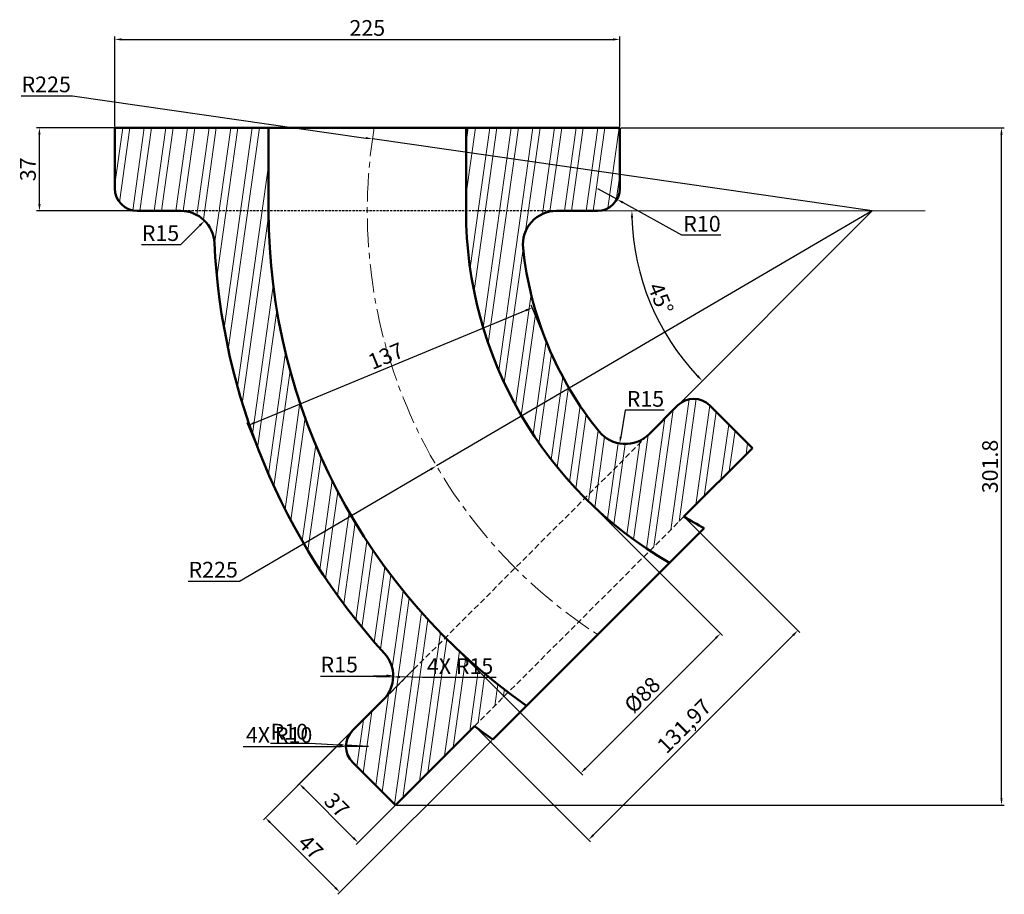
# Model space of a CAD drawing. Units: millimetres. Extents: x 315 to 754, y 170 to 559.
import ezdxf

# ---------------------------------------------------------------- set-up
doc = ezdxf.new("R2010")
doc.units = ezdxf.units.MM
doc.header["$LTSCALE"] = 0.4
doc.linetypes.add('CENTER', pattern=[50.8, 31.75, -6.35, 6.35, -6.35])
doc.linetypes.add('HIDDEN', pattern=[9.525, 6.35, -3.175])
for name, color, linetype, lineweight in [('M-CNTR', 4, 'CENTER', 18), ('M-CONS', 8, 'Continuous', 13), ('M-DIMS', 2, 'Continuous', 25), ('M-HATC', 9, 'Continuous', 18), ('M-HIDN', 3, 'HIDDEN', 25), ('M-OUTL', 7, 'Continuous', 50)]:
    doc.layers.add(name, color=color, linetype=linetype, lineweight=lineweight)
doc.styles.get("Standard").update_dxf_attribs({"font": 'arial.ttf'})
doc.dimstyles.new('ISO-25', dxfattribs={"dimtxt": 7, "dimasz": 3, "dimexe": 1.25, "dimexo": 0.625, "dimtad": 1, "dimtoh": 1, "dimtxsty": 'Standard', "dimcen": 2.5, "dimadec": 0, "dimazin": 0, "dimtfac": 1, "dimtmove": 0, "dimatfit": 3, "dimfxl": 1, "dimarcsym": 0})

# ---------------------------------------------------------------- blocks, each defined once
blk = doc.blocks.new('*D1')
at = {"layer": 'Defpoints', "color": 0, "ltscale": 0.4, "transparency": 16777216}
for p in [(582.55, 550.47), (357.55, 511.07), (582.55, 511.07)]:
    blk.add_point(p, dxfattribs=at)
at = {"layer": 'M-DIMS', "color": 0, "lineweight": -2, "ltscale": 0.4, "transparency": 16777216}
for p, q in [((357.55, 511.69), (357.55, 551.72)), ((360.55, 550.47), (579.55, 550.47)), ((582.55, 511.69), (582.55, 551.72))]:
    blk.add_line(p, q, dxfattribs=at)
at = {"layer": 'M-DIMS', "color": 0, "ltscale": 0.4, "transparency": 16777216}
for points in [[(360.55, 550.97), (360.55, 549.97), (357.55, 550.47)], [(579.55, 550.97), (579.55, 549.97), (582.55, 550.47)]]:
    blk.add_solid(points, dxfattribs=at)
at = {"layer": 'M-DIMS', "color": 0, "ltscale": 0.4, "transparency": 16777216, "insert": (470.05, 554.67), "char_height": 7, "attachment_point": 5}
blk.add_mtext('225', dxfattribs=at)
blk = doc.blocks.new('*D2')
at = {"layer": 'Defpoints', "color": 0, "ltscale": 0.4, "transparency": 16777216}
for p in [(323.97, 511.07), (377.23, 511.07), (377.23, 474.07)]:
    blk.add_point(p, dxfattribs=at)
at = {"layer": 'M-DIMS', "color": 0, "lineweight": -2, "ltscale": 0.4, "transparency": 16777216}
for p, q in [((376.61, 511.07), (322.72, 511.07)), ((323.97, 477.07), (323.97, 508.07)), ((376.61, 474.07), (322.72, 474.07))]:
    blk.add_line(p, q, dxfattribs=at)
at = {"layer": 'M-DIMS', "color": 0, "ltscale": 0.4, "transparency": 16777216}
for points in [[(323.47, 508.07), (324.47, 508.07), (323.97, 511.07)], [(323.47, 477.07), (324.47, 477.07), (323.97, 474.07)]]:
    blk.add_solid(points, dxfattribs=at)
at = {"layer": 'M-DIMS', "color": 0, "ltscale": 0.4, "transparency": 16777216, "insert": (319.76, 492.57), "char_height": 7, "attachment_point": 5, "rotation": 90}
blk.add_mtext('37', dxfattribs=at)
blk = doc.blocks.new('*D3')
at = {"layer": 'Defpoints', "color": 0, "ltscale": 0.4, "transparency": 16777216}
for p in [(543.54, 430.9), (550.46, 414.18), (423.89, 361.75)]:
    blk.add_point(p, dxfattribs=at)
at = {"layer": 'M-DIMS', "color": 0, "lineweight": -2, "ltscale": 0.4, "transparency": 16777216}
for p, q in [((550.23, 414.75), (543.06, 432.05)), ((419.74, 379.62), (540.77, 429.75)), ((423.65, 362.33), (416.49, 379.63))]:
    blk.add_line(p, q, dxfattribs=at)
at = {"layer": 'M-DIMS', "color": 0, "ltscale": 0.4, "transparency": 16777216}
for points in [[(540.58, 430.21), (540.96, 429.29), (543.54, 430.9)], [(419.55, 380.08), (419.93, 379.16), (416.97, 378.47)]]:
    blk.add_solid(points, dxfattribs=at)
at = {"layer": 'M-DIMS', "color": 0, "ltscale": 0.4, "transparency": 16777216, "insert": (478.64, 408.57), "char_height": 7, "attachment_point": 5, "rotation": 22.5}
blk.add_mtext('137', dxfattribs=at)
blk = doc.blocks.new('*D4')
at = {"layer": 'Defpoints', "color": 0, "ltscale": 0.4, "transparency": 16777216}
for p in [(567.07, 346.08), (627.38, 285.76), (504.84, 283.86)]:
    blk.add_point(p, dxfattribs=at)
at = {"layer": 'M-DIMS', "color": 0, "lineweight": -2, "ltscale": 0.4, "transparency": 16777216}
for p, q in [((567.51, 345.64), (628.27, 284.88)), ((505.28, 283.41), (566.04, 222.65)), ((567.28, 225.66), (625.26, 283.64))]:
    blk.add_line(p, q, dxfattribs=at)
at = {"layer": 'M-DIMS', "color": 0, "ltscale": 0.4, "transparency": 16777216}
for points in [[(624.91, 284), (625.61, 283.29), (627.38, 285.76)], [(566.92, 226.01), (567.63, 225.31), (565.16, 223.54)]]:
    blk.add_solid(points, dxfattribs=at)
at = {"layer": 'M-DIMS', "color": 0, "ltscale": 0.4, "transparency": 16777216, "insert": (593.16, 257.76), "char_height": 7, "attachment_point": 5, "rotation": 45}
blk.add_mtext('%%C88', dxfattribs=at)
blk = doc.blocks.new('*D5')
at = {"layer": 'Defpoints', "color": 0, "ltscale": 0.4, "transparency": 16777216}
for p in [(611.14, 337.83), (661.89, 287.08), (517.83, 244.52)]:
    blk.add_point(p, dxfattribs=at)
at = {"layer": 'M-DIMS', "color": 0, "lineweight": -2, "ltscale": 0.4, "transparency": 16777216}
for p, q in [((611.59, 337.39), (662.78, 286.2)), ((570.7, 195.89), (659.77, 284.96)), ((518.27, 244.08), (569.46, 192.88))]:
    blk.add_line(p, q, dxfattribs=at)
at = {"layer": 'M-DIMS', "color": 0, "ltscale": 0.4, "transparency": 16777216}
for points in [[(659.42, 285.32), (660.13, 284.61), (661.89, 287.08)], [(570.35, 196.24), (571.05, 195.54), (568.58, 193.77)]]:
    blk.add_solid(points, dxfattribs=at)
at = {"layer": 'M-DIMS', "color": 0, "ltscale": 0.4, "transparency": 16777216, "insert": (611.82, 243.84), "char_height": 7, "attachment_point": 5, "rotation": 45}
blk.add_mtext('131,97', dxfattribs=at)
blk = doc.blocks.new('*D6')
at = {"layer": 'Defpoints', "color": 0, "ltscale": 0.4, "transparency": 16777216}
for p in [(477.17, 256.18), (503.33, 230.02), (465.92, 192.61)]:
    blk.add_point(p, dxfattribs=at)
at = {"layer": 'M-DIMS', "color": 0, "lineweight": -2, "ltscale": 0.4, "transparency": 16777216}
for p, q in [((476.73, 255.74), (438.87, 217.89)), ((502.89, 229.58), (465.03, 191.72)), ((441.88, 216.65), (463.8, 194.73))]:
    blk.add_line(p, q, dxfattribs=at)
at = {"layer": 'M-DIMS', "color": 0, "ltscale": 0.4, "transparency": 16777216}
for points in [[(442.23, 217), (441.52, 216.29), (439.75, 218.77)], [(464.15, 195.08), (463.44, 194.37), (465.92, 192.61)]]:
    blk.add_solid(points, dxfattribs=at)
at = {"layer": 'M-DIMS', "color": 0, "ltscale": 0.4, "transparency": 16777216, "insert": (455.81, 208.66), "char_height": 7, "attachment_point": 5, "rotation": 315}
blk.add_mtext('37', dxfattribs=at)
blk = doc.blocks.new('*D7')
at = {"layer": 'Defpoints', "color": 0, "ltscale": 0.4, "transparency": 16777216}
for p in [(492.7, 271.72), (525.94, 238.48), (424.63, 203.64)]:
    blk.add_point(p, dxfattribs=at)
at = {"layer": 'M-DIMS', "color": 0, "lineweight": -2, "ltscale": 0.4, "transparency": 16777216}
for p, q in [((492.26, 271.28), (423.74, 202.76)), ((525.49, 238.04), (456.98, 169.53)), ((455.74, 172.53), (426.75, 201.52))]:
    blk.add_line(p, q, dxfattribs=at)
at = {"layer": 'M-DIMS', "color": 0, "ltscale": 0.4, "transparency": 16777216}
for points in [[(427.1, 201.88), (426.4, 201.17), (424.63, 203.64)], [(456.09, 172.88), (455.39, 172.18), (457.86, 170.41)]]:
    blk.add_solid(points, dxfattribs=at)
at = {"layer": 'M-DIMS', "color": 0, "ltscale": 0.4, "transparency": 16777216, "insert": (444.16, 189.94), "char_height": 7, "attachment_point": 5, "rotation": 315}
blk.add_mtext('47', dxfattribs=at)
blk = doc.blocks.new('*D8')
at = {"layer": 'Defpoints', "color": 0, "ltscale": 0.4, "transparency": 16777216}
for p in [(572.55, 484.07), (581.3, 479.22)]:
    blk.add_point(p, dxfattribs=at)
at = {"layer": 'M-DIMS', "color": 0, "lineweight": -2, "ltscale": 0.4, "transparency": 16777216}
for p, q in [((572.55, 484.07), (581.3, 479.22)), ((610.17, 463.22), (583.92, 477.77)), ((627.5, 463.22), (610.17, 463.22))]:
    blk.add_line(p, q, dxfattribs=at)
at = {"layer": 'M-DIMS', "color": 0, "ltscale": 0.4, "transparency": 16777216}
blk.add_solid([(584.16, 478.2), (583.68, 477.33), (581.3, 479.22)], dxfattribs=at)
at = {"layer": 'M-DIMS', "color": 0, "ltscale": 0.4, "transparency": 16777216, "insert": (619.15, 467.42), "char_height": 7, "attachment_point": 5}
blk.add_mtext('R10', dxfattribs=at)
blk = doc.blocks.new('*D9')
at = {"layer": 'Defpoints', "color": 0, "ltscale": 0.4, "transparency": 16777216}
for p in [(584.95, 385.18), (582.45, 370.39)]:
    blk.add_point(p, dxfattribs=at)
at = {"layer": 'M-DIMS', "color": 0, "lineweight": -2, "ltscale": 0.4, "transparency": 16777216}
for p, q in [((584.96, 385.2), (582.95, 373.35)), ((602.36, 385.2), (584.96, 385.2))]:
    blk.add_line(p, q, dxfattribs=at)
at = {"layer": 'M-DIMS', "color": 0, "ltscale": 0.4, "transparency": 16777216}
blk.add_solid([(582.45, 373.43), (583.44, 373.27), (582.45, 370.39)], dxfattribs=at)
at = {"layer": 'M-DIMS', "color": 0, "ltscale": 0.4, "transparency": 16777216, "insert": (593.97, 389.39), "char_height": 7, "attachment_point": 5}
blk.add_mtext('R15', dxfattribs=at)
blk = doc.blocks.new('*D10')
at = {"layer": 'Defpoints', "color": 0, "ltscale": 0.4, "transparency": 16777216}
for p in [(397.52, 469.67), (386.92, 459.07)]:
    blk.add_point(p, dxfattribs=at)
at = {"layer": 'M-DIMS', "color": 0, "lineweight": -2, "ltscale": 0.4, "transparency": 16777216}
for p, q in [((386.91, 459.06), (395.4, 467.55)), ((369.5, 459.06), (386.91, 459.06))]:
    blk.add_line(p, q, dxfattribs=at)
at = {"layer": 'M-DIMS', "color": 0, "ltscale": 0.4, "transparency": 16777216}
blk.add_solid([(395.05, 467.91), (395.76, 467.2), (397.52, 469.67)], dxfattribs=at)
at = {"layer": 'M-DIMS', "color": 0, "ltscale": 0.4, "transparency": 16777216, "insert": (377.89, 463.26), "char_height": 7, "attachment_point": 5}
blk.add_mtext('R15', dxfattribs=at)
blk = doc.blocks.new('*D11')
at = {"layer": 'Defpoints', "color": 0, "ltscale": 0.4, "transparency": 16777216}
for p in [(695.05, 474.07), (500.86, 360.42)]:
    blk.add_point(p, dxfattribs=at)
at = {"layer": 'M-DIMS', "color": 0, "lineweight": -2, "ltscale": 0.4, "transparency": 16777216}
for p, q in [((695.05, 474.07), (500.86, 360.42)), ((413.12, 309.07), (498.27, 358.9)), ((390.28, 309.07), (413.12, 309.07))]:
    blk.add_line(p, q, dxfattribs=at)
at = {"layer": 'M-DIMS', "color": 0, "ltscale": 0.4, "transparency": 16777216}
blk.add_solid([(498.02, 359.33), (498.53, 358.47), (500.86, 360.42)], dxfattribs=at)
at = {"layer": 'M-DIMS', "color": 0, "ltscale": 0.4, "transparency": 16777216, "insert": (401.39, 313.27), "char_height": 7, "attachment_point": 5}
blk.add_mtext('R225', dxfattribs=at)
blk = doc.blocks.new('*D12')
at = {"layer": 'Defpoints', "color": 0, "ltscale": 0.4, "transparency": 16777216}
for p in [(466.56, 266.79), (481.56, 267)]:
    blk.add_point(p, dxfattribs=at)
at = {"layer": 'M-DIMS', "color": 0, "lineweight": -2, "ltscale": 0.4, "transparency": 16777216}
for p, q in [((449.14, 266.79), (466.55, 266.79)), ((466.55, 266.79), (478.56, 266.96))]:
    blk.add_line(p, q, dxfattribs=at)
at = {"layer": 'M-DIMS', "color": 0, "ltscale": 0.4, "transparency": 16777216}
blk.add_solid([(478.55, 267.46), (478.57, 266.46), (481.56, 267)], dxfattribs=at)
at = {"layer": 'M-DIMS', "color": 0, "ltscale": 0.4, "transparency": 16777216, "insert": (457.53, 270.99), "char_height": 7, "attachment_point": 5}
blk.add_mtext('R15', dxfattribs=at)
blk = doc.blocks.new('*D13')
at = {"layer": 'Defpoints', "color": 0, "ltscale": 0.4, "transparency": 16777216}
for p in [(460.56, 235.98), (470.55, 235.42)]:
    blk.add_point(p, dxfattribs=at)
at = {"layer": 'M-DIMS', "color": 0, "lineweight": -2, "ltscale": 0.4, "transparency": 16777216}
for p, q in [((426.96, 236.9), (444.29, 236.9)), ((444.29, 236.9), (457.57, 236.15)), ((470.55, 235.42), (460.56, 235.98))]:
    blk.add_line(p, q, dxfattribs=at)
at = {"layer": 'M-DIMS', "color": 0, "ltscale": 0.4, "transparency": 16777216}
blk.add_solid([(457.59, 236.65), (457.54, 235.65), (460.56, 235.98)], dxfattribs=at)
at = {"layer": 'M-DIMS', "color": 0, "ltscale": 0.4, "transparency": 16777216, "insert": (435.31, 241.1), "char_height": 7, "attachment_point": 5}
blk.add_mtext('R10', dxfattribs=at)
blk = doc.blocks.new('*D14')
at = {"layer": 'Defpoints', "color": 0, "ltscale": 0.4, "transparency": 16777216}
for p in [(563.45, 474.07), (695.05, 474.07), (718.61, 474.07), (591.59, 446.35), (602, 381.01)]:
    blk.add_point(p, dxfattribs=at)
at = {"layer": 'M-DIMS', "color": 0, "lineweight": -2, "ltscale": 0.4, "transparency": 16777216}
blk.add_arc((695.05, 474.07), 107.11, 181.6048, 223.3952, dxfattribs=at)
at = {"layer": 'M-DIMS', "color": 0, "ltscale": 0.4, "transparency": 16777216}
for points in [[(587.49, 471.06), (588.49, 471.07), (587.94, 474.07)], [(617.58, 400.83), (616.86, 400.13), (619.31, 398.33)]]:
    blk.add_solid(points, dxfattribs=at)
at = {"layer": 'M-DIMS', "color": 0, "ltscale": 0.4, "transparency": 16777216, "insert": (599.96, 434.68), "char_height": 7, "attachment_point": 5, "rotation": 292.5}
blk.add_mtext('45°', dxfattribs=at)
blk = doc.blocks.new('*D15')
at = {"layer": 'Defpoints', "color": 0, "ltscale": 0.4, "transparency": 16777216}
for p in [(582.55, 511.07), (752.61, 511.07), (482.57, 209.26)]:
    blk.add_point(p, dxfattribs=at)
at = {"layer": 'M-DIMS', "color": 0, "lineweight": -2, "ltscale": 0.4, "transparency": 16777216}
for p, q in [((583.18, 511.07), (753.86, 511.07)), ((752.61, 212.26), (752.61, 508.07)), ((483.19, 209.26), (753.86, 209.26))]:
    blk.add_line(p, q, dxfattribs=at)
at = {"layer": 'M-DIMS', "color": 0, "ltscale": 0.4, "transparency": 16777216}
for points in [[(752.11, 508.07), (753.11, 508.07), (752.61, 511.07)], [(752.11, 212.26), (753.11, 212.26), (752.61, 209.26)]]:
    blk.add_solid(points, dxfattribs=at)
at = {"layer": 'M-DIMS', "color": 0, "ltscale": 0.4, "transparency": 16777216, "insert": (748.41, 360.16), "char_height": 7, "attachment_point": 5, "rotation": 90}
blk.add_mtext('301.8', dxfattribs=at)
blk = doc.blocks.new('*D16')
at = {"layer": 'Defpoints', "color": 0, "ltscale": 0.4, "transparency": 16777216}
for p in [(466.56, 266.79), (481.56, 266.43)]:
    blk.add_point(p, dxfattribs=at)
at = {"layer": 'M-DIMS', "color": 0, "lineweight": -2, "ltscale": 0.4, "transparency": 16777216}
for p, q in [((466.56, 266.79), (481.56, 266.43)), ((494.7, 266.11), (484.56, 266.36)), ((527.43, 266.11), (494.7, 266.11))]:
    blk.add_line(p, q, dxfattribs=at)
at = {"layer": 'M-DIMS', "color": 0, "ltscale": 0.4, "transparency": 16777216}
blk.add_solid([(484.57, 266.86), (484.54, 265.86), (481.56, 266.43)], dxfattribs=at)
at = {"layer": 'M-DIMS', "color": 0, "ltscale": 0.4, "transparency": 16777216, "insert": (511.38, 270.31), "char_height": 7, "attachment_point": 5}
blk.add_mtext('4X R15', dxfattribs=at)
blk = doc.blocks.new('*D17')
at = {"layer": 'Defpoints', "color": 0, "ltscale": 0.4, "transparency": 16777216}
for p in [(460.55, 235.42), (470.55, 235.42)]:
    blk.add_point(p, dxfattribs=at)
at = {"layer": 'M-DIMS', "color": 0, "lineweight": -2, "ltscale": 0.4, "transparency": 16777216}
for p, q in [((414.75, 235.42), (447.4, 235.42)), ((447.4, 235.42), (457.55, 235.42)), ((470.55, 235.42), (460.55, 235.42))]:
    blk.add_line(p, q, dxfattribs=at)
at = {"layer": 'M-DIMS', "color": 0, "ltscale": 0.4, "transparency": 16777216}
blk.add_solid([(457.55, 235.92), (457.55, 234.92), (460.55, 235.42)], dxfattribs=at)
at = {"layer": 'M-DIMS', "color": 0, "ltscale": 0.4, "transparency": 16777216, "insert": (430.76, 239.62), "char_height": 7, "attachment_point": 5}
blk.add_mtext('4X R10', dxfattribs=at)
blk = doc.blocks.new('*D18')
at = {"layer": 'Defpoints', "color": 0, "ltscale": 0.4, "transparency": 16777216}
for p in [(472.34, 506.1), (695.05, 474.07)]:
    blk.add_point(p, dxfattribs=at)
at = {"layer": 'M-DIMS', "color": 0, "lineweight": -2, "ltscale": 0.4, "transparency": 16777216}
for p, q in [((315.88, 525.32), (338.72, 525.32)), ((338.72, 525.32), (469.37, 506.53)), ((695.05, 474.07), (472.34, 506.1))]:
    blk.add_line(p, q, dxfattribs=at)
at = {"layer": 'M-DIMS', "color": 0, "ltscale": 0.4, "transparency": 16777216}
blk.add_solid([(469.45, 507.02), (469.3, 506.03), (472.34, 506.1)], dxfattribs=at)
at = {"layer": 'M-DIMS', "color": 0, "ltscale": 0.4, "transparency": 16777216, "insert": (326.99, 529.52), "char_height": 7, "attachment_point": 5}
blk.add_mtext('R225', dxfattribs=at)

msp = doc.modelspace()

# ---------------------------------------------------------------- hatches: boundary and pattern name
at = {"layer": 'M-HATC', "ltscale": 0.4}
h = msp.add_hatch(dxfattribs=at)
h.set_pattern_fill('ANSI32', color=256, angle=37)
h.set_pattern_definition([(82, (-1722.207, -282.083), (-9.432303, 1.325624), []), (82, (-1718.621, -279.38), (-9.432303, 1.325624), [])])
h.paths.add_polyline_path([(426.052, 511.067), (357.552, 511.067), (357.552, 484.067, 0.4142136), (367.552, 474.067), (386.916, 474.067), (426.052, 474.067)])
h.paths.add_polyline_path([(426.052, 474.067), (386.916, 474.067, -0.4000375), (401.899, 459.796, 0.1737461), (477.67, 276.867, -0.4000375), (477.167, 256.182), (504.84, 283.855, -0.1989124)])
h.paths.add_polyline_path([(517.829, 244.519), (532.811, 259.5, -0.0345097), (504.84, 283.855), (477.167, 256.182), (463.474, 242.489, 0.4142136), (463.474, 228.347), (482.566, 209.255)])
h.paths.add_polyline_path([(582.552, 511.067), (514.052, 511.067), (514.052, 474.067), (554.349, 474.067), (572.552, 474.067, 0.4142136), (582.552, 484.067)])
h.paths.add_polyline_path([(539.433, 457.477, -0.4456742), (554.349, 474.067), (514.052, 474.067, 0.1989124), (567.065, 346.081), (595.56, 374.575, -0.4456742), (573.282, 375.759, -0.1442341)])
h.paths.add_polyline_path([(641.665, 368.354), (622.573, 387.446, 0.4142136), (608.431, 387.446), (595.56, 374.575), (567.065, 346.081, 0.0515133), (595.931, 322.62), (611.144, 337.834)])

# ---------------------------------------------------------------- linework, layer by layer
at = {"layer": 'M-CNTR'}
msp.add_arc((695.052, 474.067), 225, 170.53504, 237.05725, dxfattribs=at)
at = {"layer": 'M-CONS', "ltscale": 0.4}
for p, q in [((563.45, 474.067), (718.613, 474.067)), ((695.052, 474.067), (601.995, 381.011))]:
    msp.add_line(p, q, dxfattribs=at)
at = {"layer": 'M-HIDN', "ltscale": 0.4}
msp.add_line((554.349, 474.067), (386.916, 474.067), dxfattribs=at)
at = {"layer": 'M-HIDN'}
for p, q in [((608.431, 387.446), (477.167, 256.182)), ((611.144, 337.834), (517.829, 244.519))]:
    msp.add_line(p, q, dxfattribs=at)
at = {"layer": 'M-OUTL'}
for p, q in [((357.552, 511.067), (582.552, 511.067)), ((357.552, 484.067), (357.552, 511.067)), ((582.552, 484.067), (582.552, 511.067)), ((367.552, 474.067), (386.916, 474.067)), ((554.349, 474.067), (572.552, 474.067)), ((595.56, 374.575), (608.431, 387.446)), ((622.573, 387.446), (641.665, 368.354)), ((641.665, 368.354), (611.144, 337.834)), ((620.14, 332.687), (525.936, 238.483)), ((463.474, 228.347), (482.566, 209.255))]:
    msp.add_line(p, q, dxfattribs=at)
at = {"layer": 'M-OUTL', "ltscale": 0.4}
for p, q in [((426.052, 474.067), (426.052, 511.067)), ((514.052, 474.067), (514.052, 511.067)), ((477.167, 256.182), (463.474, 242.489)), ((517.829, 244.519), (482.566, 209.255))]:
    msp.add_line(p, q, dxfattribs=at)
at = {"layer": 'M-OUTL'}
for centre, radius, start, end in [((367.552, 484.067), 10, 180, 270), ((572.552, 484.067), 10, 270, 0), ((386.916, 459.067), 15, 2.78696, 90), ((695.052, 474.067), 269, 180, 235.06243), ((695.052, 474.067), 181, 180, 240.05039), ((554.349, 459.067), 15, 90, 186.08519), ((695.052, 474.067), 293.5, 182.78696, 222.21304), ((695.052, 474.067), 156.5, 186.08519, 218.91481), ((615.502, 380.375), 10, 45, 135), ((584.953, 385.182), 15, 218.91481, 315), ((695.052, 474.067), 160, 238.37068, 242.0826), ((466.561, 266.789), 15, 315, 42.21304), ((470.545, 235.418), 10, 135, 225), ((695.052, 474.067), 290, 232.33013, 234.32701)]:
    msp.add_arc(centre, radius, start, end, dxfattribs=at)

# ---------------------------------------------------------------- dimensions: what is measured, and where the dimension line sits
at = {"layer": 'M-DIMS', "ltscale": 0.4}
for p1, p2, distance, picture, middle in [((357.552, 511.067), (582.552, 511.067), 39.4, '*D1', (470.052, 554.666)), ((377.234, 474.067), (377.234, 511.067), 53.268, '*D2', (319.765, 492.567)), ((423.893, 361.749), (550.464, 414.177), 18.099, '*D3', (478.645, 408.566)), ((517.829, 244.519), (611.144, 337.834), -71.772, '*D5', (611.821, 243.842)), ((525.936, 238.483), (492.702, 271.717), 96.271, '*D7', (444.161, 189.943)), ((477.167, 256.182), (503.33, 230.02), -52.911, '*D6', (455.806, 208.658))]:
    dim = msp.add_aligned_dim(p1=p1, p2=p2, distance=distance, dimstyle='ISO-25', override={"dimclrd": 0, "dimclre": 0, "dimclrt": 0}, dxfattribs=at)
    dim.commit()
    dim.dimension.update_dxf_attribs({"geometry": picture, "text_midpoint": middle})
for center, mpoint, override, picture, middle in [((695.052, 474.067), (472.344, 506.101), {"dimdec": 0, "dimlfac": 1, "dimrnd": 0, "dimzin": 0, "dimdsep": 46, "dimlunit": 2}, '*D18', (338.719, 525.321)), ((572.552, 484.067), (581.299, 479.22), {"dimclrd": 0, "dimclre": 0, "dimclrt": 0}, '*D8', (619.146, 463.223)), ((695.052, 474.067), (500.863, 360.419), {"dimclrd": 0, "dimclre": 0, "dimclrt": 0}, '*D11', (401.385, 309.067)), ((386.916, 459.067), (397.523, 469.673), {"dimclrd": 0, "dimclre": 0, "dimclrt": 0}, '*D10', (377.892, 459.057)), ((584.953, 385.182), (582.446, 370.393), {"dimclrd": 0, "dimclre": 0, "dimclrt": 0}, '*D9', (593.97, 385.196)), ((466.561, 266.789), (481.559, 267.004), {"dimclrd": 0, "dimclre": 0, "dimclrt": 0}, '*D12', (466.546, 266.789)), ((470.545, 235.418), (460.561, 235.983), {"dimclrd": 0, "dimclre": 0, "dimclrt": 0}, '*D13', (444.29, 236.904))]:
    dim = msp.add_radius_dim(center=center, mpoint=mpoint, dimstyle='ISO-25', override=override, dxfattribs=at)
    dim.commit()
    dim.dimension.update_dxf_attribs({"geometry": picture, "text_midpoint": middle, "dimtype": 164})
dim = msp.add_linear_dim(base=(752.613, 511.067), p1=(482.566, 209.255), p2=(582.552, 511.067), angle=90, dimstyle='ISO-25', override={"dimdec": 1, "dimlfac": 1, "dimrnd": 0, "dimzin": 0, "dimdsep": 46, "dimlunit": 2}, dxfattribs=at)
dim.commit()
dim.dimension.update_dxf_attribs({"geometry": '*D15', "text_midpoint": (748.411, 360.161)})
dim = msp.add_angular_dim_2l(base=(591.593, 446.345), line1=((695.052, 474.067), (601.995, 381.011)), line2=((563.45, 474.067), (718.613, 474.067)), dimstyle='ISO-25', override={"dimclrd": 0, "dimclre": 0, "dimclrt": 0}, dxfattribs=at)
dim.commit()
dim.dimension.update_dxf_attribs({"geometry": '*D14', "text_midpoint": (599.962, 434.68)})
dim = msp.add_aligned_dim(p1=(504.84, 283.855), p2=(567.065, 346.081), distance=-85.301, text='%%C<>', dimstyle='ISO-25', override={"dimclrd": 0, "dimclre": 0, "dimclrt": 0}, dxfattribs=at)
dim.commit()
dim.dimension.update_dxf_attribs({"geometry": '*D4', "text_midpoint": (593.162, 257.759)})
for center, mpoint, picture, middle in [((466.561, 266.789), (481.556, 266.43), '*D16', (511.376, 270.314)), ((470.545, 235.418), (460.545, 235.418), '*D17', (430.76, 239.617))]:
    dim = msp.add_radius_dim(center=center, mpoint=mpoint, text='4X <>', dimstyle='ISO-25', override={"dimdec": 0, "dimlfac": 1, "dimrnd": 0, "dimzin": 0, "dimdsep": 46, "dimlunit": 2}, dxfattribs=at)
    dim.commit()
    dim.dimension.update_dxf_attribs({"geometry": picture, "text_midpoint": middle})

doc.saveas('drawing.dxf')
